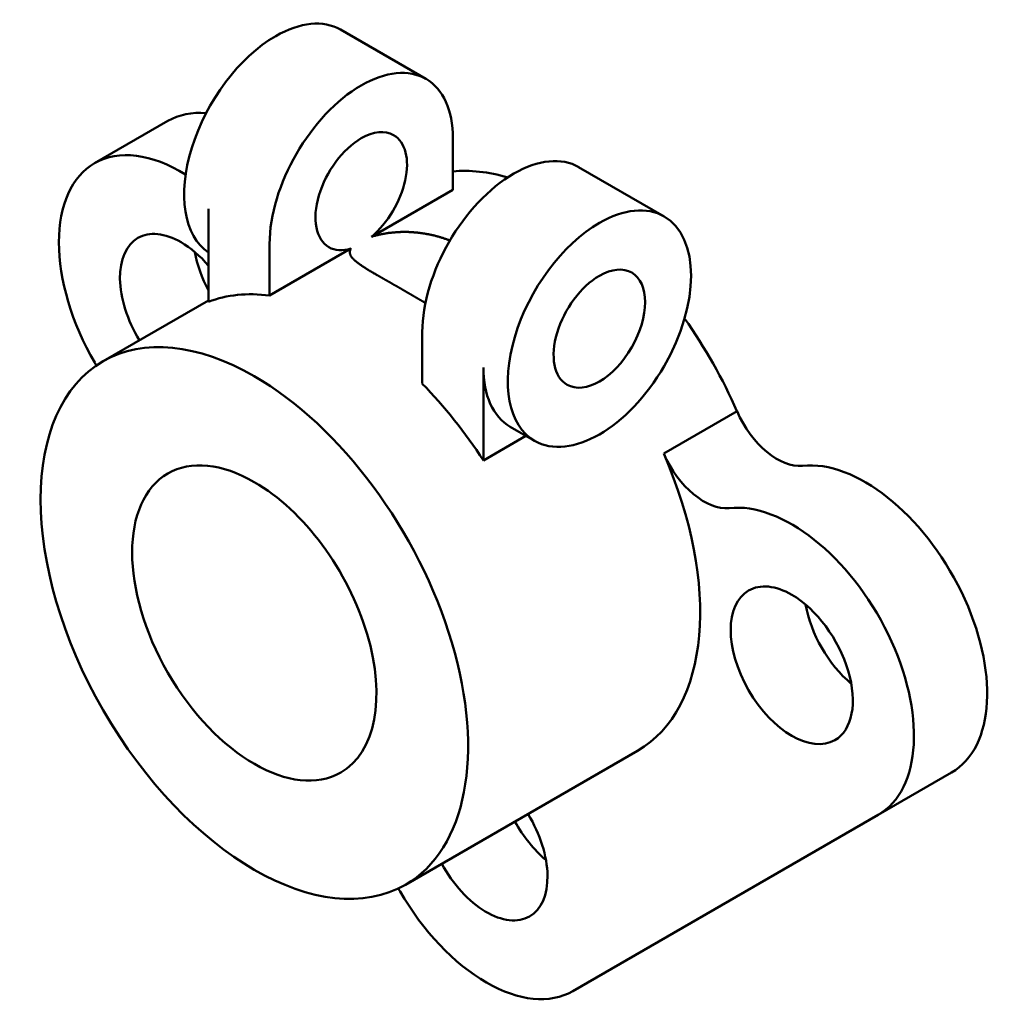
# Model space of a CAD drawing. Units: millimetres. Extents: x 1636 to 1775, y 2009 to 2149.
import ezdxf

# ---------------------------------------------------------------- set-up
doc = ezdxf.new("R2010")
doc.units = ezdxf.units.MM
doc.layers.add('M-OUTL', color=7, linetype='Continuous', lineweight=50)

msp = doc.modelspace()

# ---------------------------------------------------------------- linework, layer by layer
at = {"layer": 'M-OUTL'}
for p, q in [((1693.88, 2140.45), (1681.76, 2147.45)), ((1657.29, 2134.51), (1646.9, 2128.51)), ((1697.69, 2124.74), (1697.69, 2132.04)), ((1727.66, 2120.95), (1715.53, 2127.95)), ((1697.69, 2124.74), (1686.16, 2118.08)), ((1663.05, 2108.85), (1663.05, 2122.04)), ((1671.71, 2109.74), (1671.71, 2117.04)), ((1683.24, 2116.39), (1671.71, 2109.74)), ((1648.11, 2100.42), (1663.05, 2109.04)), ((1693.36, 2097.24), (1693.36, 2104.54)), ((1646.9, 2100.22), (1647.14, 2099.81)), ((1702.02, 2086.35), (1702.02, 2099.54)), ((1727.59, 2087.32), (1737.99, 2093.32)), ((1709.29, 2089.13), (1705.82, 2091.13)), ((1702.02, 2086.35), (1708.06, 2089.84)), ((1690.97, 2026.17), (1723.88, 2045.17)), ((1758, 2036.08), (1768.39, 2042.08)), ((1768.39, 2042.08), (1758, 2036.08)), ((1714.7, 2011.08), (1758, 2036.08)), ((1689.96, 2025.64), (1690.2, 2025.22))]:
    msp.add_line(p, q, dxfattribs=at)
for points in [[(1697.28, 2117.55), (1697.18, 2117.59), (1697.08, 2117.63), (1696.97, 2117.66), (1696.87, 2117.7), (1696.77, 2117.73), (1696.67, 2117.77), (1696.57, 2117.8), (1696.46, 2117.84), (1696.36, 2117.87), (1696.26, 2117.9), (1696.15, 2117.94), (1696.05, 2117.97), (1695.94, 2118), (1695.84, 2118.03), (1695.73, 2118.06), (1695.63, 2118.09), (1695.52, 2118.12), (1695.42, 2118.15), (1695.31, 2118.17), (1695.21, 2118.2), (1695.1, 2118.23), (1694.99, 2118.25), (1694.88, 2118.28), (1694.78, 2118.3), (1694.67, 2118.33), (1694.56, 2118.35), (1694.45, 2118.38), (1694.34, 2118.4), (1694.24, 2118.42), (1694.13, 2118.44), (1694.02, 2118.46), (1693.91, 2118.48), (1693.8, 2118.5), (1693.69, 2118.52), (1693.57, 2118.54), (1693.46, 2118.55), (1693.35, 2118.57), (1693.24, 2118.59), (1693.13, 2118.6), (1693.02, 2118.62), (1692.9, 2118.63), (1692.79, 2118.64), (1692.68, 2118.66), (1692.56, 2118.67), (1692.45, 2118.68), (1692.33, 2118.69), (1692.22, 2118.7), (1692.1, 2118.71), (1691.99, 2118.72), (1691.87, 2118.72), (1691.75, 2118.73), (1691.64, 2118.74), (1691.52, 2118.74), (1691.4, 2118.75), (1691.28, 2118.75), (1691.17, 2118.75), (1691.05, 2118.75), (1690.93, 2118.75), (1690.81, 2118.75), (1690.69, 2118.75), (1690.57, 2118.75), (1690.45, 2118.75), (1690.32, 2118.75), (1690.2, 2118.74), (1690.08, 2118.74), (1689.96, 2118.73), (1689.83, 2118.73), (1689.71, 2118.72), (1689.59, 2118.71), (1689.46, 2118.7), (1689.34, 2118.69), (1689.21, 2118.68), (1689.09, 2118.67), (1688.96, 2118.65), (1688.84, 2118.64), (1688.71, 2118.62), (1688.58, 2118.61), (1688.46, 2118.59), (1688.33, 2118.57), (1688.2, 2118.55), (1688.07, 2118.53), (1687.95, 2118.51), (1687.82, 2118.48), (1687.69, 2118.46), (1687.56, 2118.43), (1687.43, 2118.41), (1687.3, 2118.38), (1687.18, 2118.35), (1687.05, 2118.32), (1686.92, 2118.29), (1686.79, 2118.26), (1686.66, 2118.22), (1686.53, 2118.19), (1686.41, 2118.15), (1686.28, 2118.12), (1686.16, 2118.08)], [(1683.24, 2116.39), (1683.21, 2116.35), (1683.19, 2116.3), (1683.17, 2116.26), (1683.15, 2116.21), (1683.13, 2116.17), (1683.12, 2116.13), (1683.11, 2116.08), (1683.1, 2116.04), (1683.09, 2116), (1683.09, 2115.95), (1683.08, 2115.91), (1683.08, 2115.87), (1683.09, 2115.83), (1683.09, 2115.79), (1683.09, 2115.74), (1683.1, 2115.7), (1683.11, 2115.66), (1683.12, 2115.62), (1683.13, 2115.58), (1683.15, 2115.54), (1683.16, 2115.5), (1683.18, 2115.46), (1683.2, 2115.42), (1683.22, 2115.38), (1683.24, 2115.34), (1683.26, 2115.31), (1683.29, 2115.27), (1683.32, 2115.23), (1683.34, 2115.19), (1683.37, 2115.15), (1683.4, 2115.11), (1683.43, 2115.08), (1683.46, 2115.04), (1683.5, 2115), (1683.53, 2114.96), (1683.56, 2114.92), (1683.6, 2114.89), (1683.64, 2114.85), (1683.68, 2114.81), (1683.71, 2114.77), (1683.75, 2114.74), (1683.8, 2114.7), (1683.84, 2114.66), (1683.88, 2114.63), (1683.92, 2114.59), (1683.97, 2114.55), (1684.01, 2114.51), (1684.06, 2114.48), (1684.11, 2114.44), (1684.15, 2114.4), (1684.2, 2114.37), (1684.25, 2114.33), (1684.3, 2114.29), (1684.35, 2114.26), (1684.4, 2114.22), (1684.45, 2114.18), (1684.51, 2114.14), (1684.56, 2114.11), (1684.61, 2114.07), (1684.67, 2114.03), (1684.72, 2114), (1684.78, 2113.96), (1684.83, 2113.92), (1684.89, 2113.88), (1684.95, 2113.85), (1685, 2113.81), (1685.06, 2113.77), (1685.12, 2113.73), (1685.18, 2113.7), (1685.24, 2113.66), (1685.3, 2113.62), (1685.36, 2113.58), (1685.42, 2113.54), (1685.48, 2113.51), (1685.55, 2113.47), (1685.61, 2113.43), (1685.67, 2113.39), (1685.74, 2113.35), (1685.8, 2113.31), (1685.86, 2113.27), (1685.93, 2113.24), (1685.99, 2113.2), (1686.06, 2113.16), (1686.13, 2113.12), (1686.19, 2113.08), (1686.26, 2113.04), (1686.33, 2113), (1686.39, 2112.96), (1686.46, 2112.92), (1686.53, 2112.88), (1686.6, 2112.84), (1686.67, 2112.8), (1686.74, 2112.76), (1686.81, 2112.72), (1686.88, 2112.68), (1686.95, 2112.64)], [(1686.95, 2112.64), (1686.98, 2112.62), (1687.02, 2112.6), (1687.05, 2112.58), (1687.09, 2112.56), (1687.13, 2112.54), (1687.16, 2112.51), (1687.2, 2112.49), (1687.23, 2112.47), (1687.27, 2112.45), (1687.31, 2112.43), (1687.34, 2112.41), (1687.38, 2112.39), (1687.42, 2112.37), (1687.45, 2112.35), (1687.49, 2112.33), (1687.53, 2112.3), (1687.56, 2112.28), (1687.6, 2112.26), (1687.64, 2112.24), (1687.68, 2112.22), (1687.71, 2112.2), (1687.75, 2112.18), (1687.79, 2112.16), (1687.82, 2112.13), (1687.86, 2112.11), (1687.9, 2112.09), (1687.94, 2112.07), (1687.98, 2112.05), (1688.01, 2112.03), (1688.05, 2112.01), (1688.09, 2111.98), (1688.13, 2111.96), (1688.16, 2111.94), (1688.2, 2111.92), (1688.24, 2111.9), (1688.28, 2111.88), (1688.32, 2111.85), (1688.36, 2111.83), (1688.39, 2111.81), (1688.43, 2111.79), (1688.47, 2111.77), (1688.51, 2111.74), (1688.55, 2111.72), (1688.59, 2111.7), (1688.63, 2111.68), (1688.66, 2111.66), (1688.7, 2111.63), (1688.74, 2111.61), (1688.78, 2111.59), (1688.82, 2111.57), (1688.86, 2111.54), (1688.9, 2111.52), (1688.94, 2111.5), (1688.98, 2111.48), (1689.02, 2111.45), (1689.06, 2111.43), (1689.1, 2111.41), (1689.13, 2111.39), (1689.17, 2111.36), (1689.21, 2111.34), (1689.25, 2111.32), (1689.29, 2111.3), (1689.33, 2111.27), (1689.37, 2111.25), (1689.41, 2111.23), (1689.45, 2111.21), (1689.49, 2111.18), (1689.53, 2111.16), (1689.57, 2111.14), (1689.61, 2111.11), (1689.65, 2111.09), (1689.69, 2111.07), (1689.73, 2111.04), (1689.77, 2111.02), (1689.82, 2111), (1689.86, 2110.97), (1689.9, 2110.95), (1689.94, 2110.93), (1689.98, 2110.9), (1690.02, 2110.88), (1690.06, 2110.86), (1690.1, 2110.83), (1690.14, 2110.81), (1690.18, 2110.79), (1690.22, 2110.76), (1690.26, 2110.74), (1690.31, 2110.72), (1690.35, 2110.69), (1690.39, 2110.67), (1690.43, 2110.64), (1690.47, 2110.62), (1690.51, 2110.6), (1690.55, 2110.57), (1690.6, 2110.55), (1690.64, 2110.52), (1690.68, 2110.5)], [(1693.8, 2108.69), (1693.77, 2108.71), (1693.73, 2108.72), (1693.7, 2108.74), (1693.66, 2108.76), (1693.63, 2108.78), (1693.6, 2108.8), (1693.56, 2108.82), (1693.53, 2108.84), (1693.5, 2108.86), (1693.46, 2108.88), (1693.43, 2108.9), (1693.4, 2108.92), (1693.36, 2108.94), (1693.33, 2108.96), (1693.3, 2108.98), (1693.26, 2109), (1693.23, 2109.02), (1693.19, 2109.04), (1693.16, 2109.06), (1693.13, 2109.08), (1693.1, 2109.1), (1693.06, 2109.12), (1693.03, 2109.13), (1693, 2109.15), (1692.96, 2109.17), (1692.93, 2109.19), (1692.9, 2109.21), (1692.86, 2109.23), (1692.83, 2109.25), (1692.8, 2109.27), (1692.76, 2109.29), (1692.73, 2109.31), (1692.7, 2109.33), (1692.67, 2109.35), (1692.63, 2109.37), (1692.6, 2109.38), (1692.57, 2109.4), (1692.53, 2109.42), (1692.5, 2109.44), (1692.47, 2109.46), (1692.44, 2109.48), (1692.4, 2109.5), (1692.37, 2109.52), (1692.34, 2109.54), (1692.31, 2109.56), (1692.27, 2109.58), (1692.24, 2109.59), (1692.21, 2109.61), (1692.18, 2109.63), (1692.14, 2109.65), (1692.11, 2109.67), (1692.08, 2109.69), (1692.05, 2109.71), (1692.01, 2109.73), (1691.98, 2109.74), (1691.95, 2109.76), (1691.92, 2109.78), (1691.89, 2109.8), (1691.85, 2109.82), (1691.82, 2109.84), (1691.79, 2109.86), (1691.76, 2109.88), (1691.72, 2109.89), (1691.69, 2109.91), (1691.66, 2109.93), (1691.63, 2109.95), (1691.6, 2109.97), (1691.56, 2109.99), (1691.53, 2110.01), (1691.5, 2110.02), (1691.47, 2110.04), (1691.44, 2110.06), (1691.41, 2110.08), (1691.37, 2110.1), (1691.34, 2110.12), (1691.31, 2110.14), (1691.28, 2110.15), (1691.25, 2110.17), (1691.21, 2110.19), (1691.18, 2110.21), (1691.15, 2110.23), (1691.12, 2110.25), (1691.09, 2110.26), (1691.06, 2110.28), (1691.03, 2110.3), (1690.99, 2110.32), (1690.96, 2110.34), (1690.93, 2110.35), (1690.9, 2110.37), (1690.87, 2110.39), (1690.84, 2110.41), (1690.81, 2110.43), (1690.77, 2110.45), (1690.74, 2110.46), (1690.71, 2110.48), (1690.68, 2110.5)]]:
    msp.add_lwpolyline(points, dxfattribs=at)
for centre, major_axis, start_param, end_param in [((1672.57, 2131.54), (9.19, 15.91), 0, 0.785398), ((1672.57, 2131.54), (9.19, 15.91), 0.785398, 3.103779), ((1684.7, 2124.54), (9.19, 15.91), 0, 0.785398), ((1684.7, 2124.54), (9.19, 15.91), 0.785398, 2.356194), ((1684.7, 2124.54), (9.19, 15.91), 5.497787, 6.283185), ((1669.54, 2113.29), (-12.25, 21.21), 5.903077, 6.283185), ((1684.7, 2124.54), (4.59, 7.95), 0, 0.785398), ((1684.7, 2124.54), (4.59, 7.95), 0.785398, 3.141593), ((1684.7, 2124.54), (4.59, 7.95), 4.153597, 6.283185), ((1659.15, 2107.29), (-12.25, 21.21), 5.460208, 6.283185), ((1659.15, 2107.29), (-12.25, 21.21), 0, 1.5708), ((1706.35, 2112.04), (9.19, 15.91), 0, 0.785398), ((1706.35, 2112.04), (9.19, 15.91), 0.785398, 2.356194), ((1712.84, 2088.29), (21.43, -37.12), 2.602026, 2.879793), ((1718.47, 2105.04), (9.19, 15.91), 0, 0.785398), ((1718.47, 2105.04), (9.19, 15.91), 0.785398, 3.141593), ((1718.47, 2105.04), (9.19, 15.91), 3.141593, 6.283185), ((1659.15, 2107.29), (6.12, -10.61), 2.356194, 3.141593), ((1659.15, 2107.29), (6.12, -10.61), 3.141593, 4.74793), ((1659.15, 2107.29), (6.12, -10.61), 1.889429, 2.356194), ((1669.54, 2113.29), (6.12, -10.61), 4.15479, 4.649725), ((1684.7, 2124.54), (4.59, 7.95), 3.141593, 3.700384), ((1718.47, 2105.04), (4.59, 7.95), 3.141593, 6.283185), ((1718.47, 2105.04), (4.59, 7.95), 0, 0.785398), ((1718.47, 2105.04), (4.59, 7.95), 0.785398, 3.141593), ((1682.53, 2070.79), (21.43, -37.12), 2.721402, 3.054417), ((1712.84, 2088.29), (21.43, -37.12), 1.377829, 1.732464), ((1669.54, 2063.29), (21.43, -37.12), 2.356194, 3.141593), ((1669.54, 2063.29), (21.43, -37.12), 3.141593, 6.283185), ((1715.01, 2107.04), (9.19, 15.91), 2.356194, 3.141593), ((1669.54, 2063.29), (21.43, -37.12), 0, 2.356194), ((1682.53, 2070.79), (21.43, -37.12), 1.657972, 1.990987), ((1743.72, 2094.51), (4.9, -8.49), 4.524377, 6.035892), ((1702.45, 2082.29), (21.43, -37.12), 0, 1.377829), ((1733.32, 2088.51), (4.9, -8.49), 4.524377, 6.035892), ((1669.54, 2063.29), (12.25, -21.21), 2.356194, 3.141593), ((1756.14, 2063.29), (-12.25, 21.21), 3.141593, 6.035886), ((1669.54, 2063.29), (12.25, -21.21), 3.141593, 6.283185), ((1669.54, 2063.29), (12.25, -21.21), 0, 2.356194), ((1745.75, 2057.29), (-12.25, 21.21), 3.141593, 6.035886), ((1745.75, 2057.29), (6.12, -10.61), 2.356194, 3.141593), ((1745.75, 2057.29), (6.12, -10.61), 3.141593, 6.283185), ((1745.75, 2057.29), (6.12, -10.61), 0, 2.356194), ((1756.14, 2063.29), (6.12, -10.61), 4.15479, 5.269988), ((1756.14, 2063.29), (-12.25, 21.21), 3.141589, 3.141593), ((1702.45, 2032.29), (6.12, -10.61), 0, 1.606338), ((1712.84, 2038.29), (6.12, -10.61), 4.676848, 5.269988), ((1745.75, 2057.29), (-12.25, 21.21), 3.141589, 3.141593), ((1702.45, 2032.29), (6.12, -10.61), 4.676848, 6.283185), ((1702.45, 2032.29), (-12.25, 21.21), 1.57079, 3.141593), ((1712.84, 2038.29), (-12.25, 21.21), 3.141587, 3.141593), ((1702.45, 2032.29), (-12.25, 21.21), 3.141593, 3.141599)]:
    msp.add_ellipse(centre, major_axis=major_axis, ratio=0.57735, start_param=start_param, end_param=end_param, dxfattribs=at)

doc.saveas('drawing.dxf')
